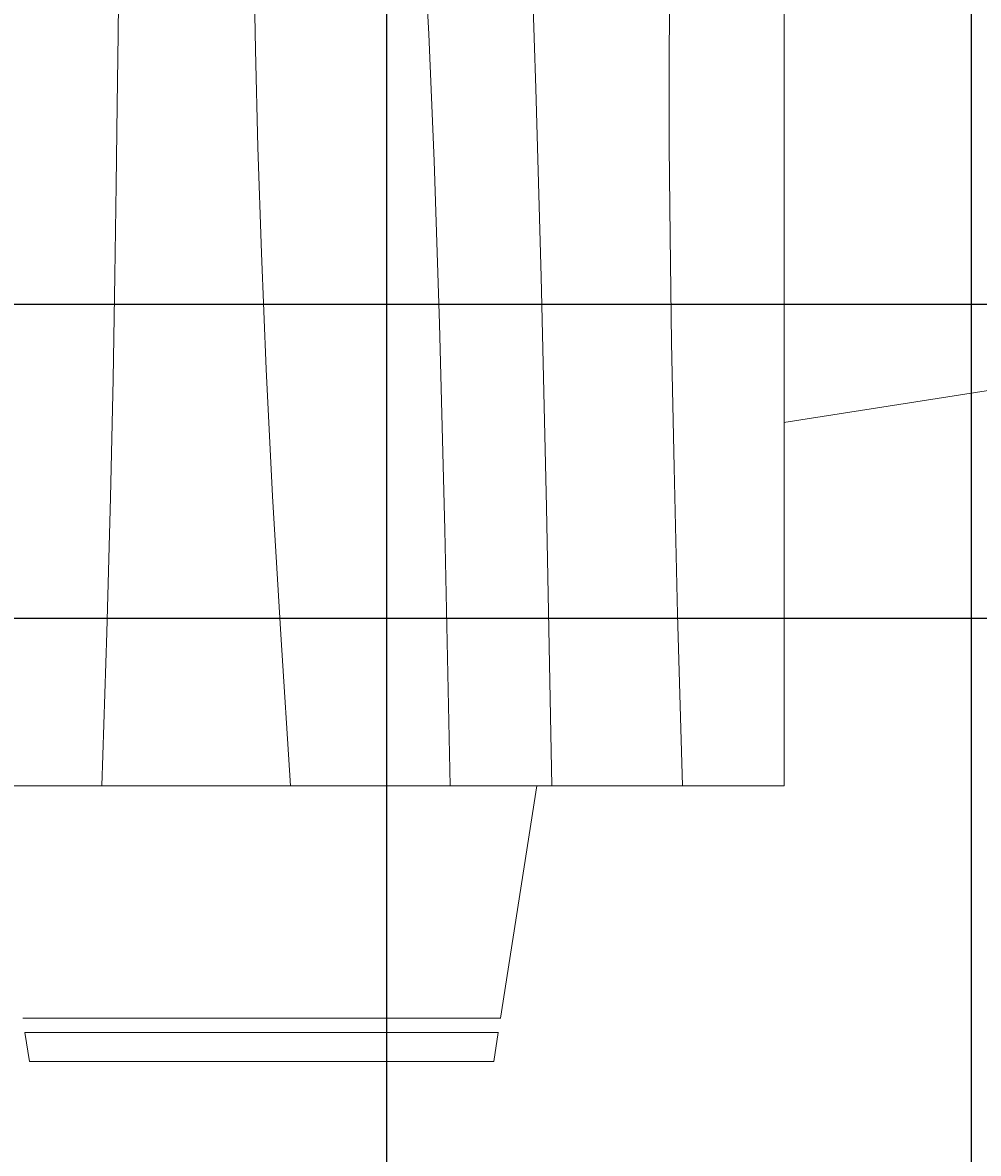
# Model space of a CAD drawing. Units: feet. Extents: x 1654 to 2985, y 1348 to 2230.
# Tile 26 of 53: x 1985 to 2014, y 1785 to 1820. Entities that reach past the tile are written whole.
import ezdxf

# ---------------------------------------------------------------- set-up
doc = ezdxf.new("R2010")
doc.units = ezdxf.units.FT
doc.layers.add('A-ANNO-DIMS', color=2, linetype='Continuous', lineweight=18)
doc.layers.add('A-FURN', color=8, linetype='Continuous', lineweight=13)
doc.styles.get("Standard").update_dxf_attribs({"font": 'arial.ttf'})
doc.dimstyles.get("Standard").update_dxf_attribs({"dimtxt": 0.18, "dimasz": 0.18, "dimexe": 0.18, "dimexo": 0.0625, "dimgap": 0.09, "dimtad": 0, "dimtih": 1, "dimtoh": 1, "dimdec": 4, "dimzin": 0, "dimdsep": 46, "dimtxsty": 'Standard', "dimcen": 0.09, "dimadec": 0, "dimazin": 0, "dimtfac": 1, "dimtdec": 4, "dimtofl": 0, "dimtmove": 0, "dimatfit": 3, "dimfxl": 1, "dimtolj": 1, "dimtzin": 0, "dimarcsym": 0})

# ---------------------------------------------------------------- blocks, each defined once
blk = doc.blocks.new('Dining Set - 36 x 72 in.')
for p, q in [((-36, 18), (-36, -18)), ((-44, 8.23041), (-44, -8.23915)), ((-45.5, 8), (-44.5004, 8.15617)), ((-45.5, 8), (-45.5, -8)), ((-44.5, -8.15843), (-44.5, 8.15338)), ((-44.4997, -8.15631), (-45.5, -8)), ((-35.9976, -9.48476), (-43.9993, -8.2345)), ((-36, -18), (36, -18)), ((-22.2343, -26.0006), (-23.4847, -17.99762))]:
    blk.add_line(p, q)
for points in [[(-36, 5.5), (-30.7157, 5.3348), (-26.069, 5.20963), (-21.9946, 5.11767), (-18.4271, 5.05208), (-15.3009, 5.00602), (-12.5508, 4.97265), (-10.1112, 4.94515), (-7.9167, 4.91666)], [(-36, -1), (-30.7915, -0.6591), (-26.0195, -0.38216), (-21.6519, -0.16284), (-17.6563, 0.00521), (-14.0005, 0.12833), (-10.6523, 0.21289), (-7.5796, 0.26522)], [(-36, -6.5), (-27.1843, -6.31267), (-20.084, -6.1263), (-14.469, -5.9419), (-10.1094, -5.76042), (-6.7752, -5.58285)], [(-36, -10), (-26.4022, -9.81299), (-18.4675, -9.62891), (-11.9839, -9.45069), (-6.7396, -9.28125)], [(-36, -14.5), (-30.0881, -14.33513), (-25.0332, -14.21224), (-20.7312, -14.12647), (-17.0781, -14.07292), (-13.97, -14.04671), (-11.3027, -14.04297), (-8.9724, -14.05681)]]:
    blk.add_lwpolyline(points)
blk = doc.blocks.new('*D91')
at = {"layer": 'A-ANNO-DIMS', "color": 0, "lineweight": -2, "transparency": 16777216}
for p, q in [((1852.155, 1801.468), (2242.272, 1801.468)), ((2242.092, 1801.288), (2242.092, 1776.544)), ((2242.092, 1751.435), (2242.092, 1776.18)), ((1852.155, 1751.255), (2242.272, 1751.255))]:
    blk.add_line(p, q, dxfattribs=at)
at = {"layer": 'A-ANNO-DIMS', "color": 0, "transparency": 16777216}
for points in [[(2242.062, 1801.288), (2242.122, 1801.288), (2242.092, 1801.468)], [(2242.062, 1751.435), (2242.122, 1751.435), (2242.092, 1751.255)]]:
    blk.add_solid(points, dxfattribs=at)
at = {"layer": 'Defpoints', "color": 0, "transparency": 16777216}
for p in [(1852.092, 1801.468), (2242.092, 1801.468), (1852.092, 1751.255)]:
    blk.add_point(p, dxfattribs=at)
at = {"layer": 'A-ANNO-DIMS', "color": 0, "transparency": 16777216, "insert": (2242.092, 1776.362), "char_height": 0.18, "attachment_point": 5}
blk.add_mtext('\\A1;50.21', dxfattribs=at)
blk = doc.blocks.new('*D98')
at = {"layer": 'A-ANNO-DIMS', "color": 0, "lineweight": -2, "transparency": 16777216}
for p, q in [((2061.03, 1811.081), (1811.912, 1811.081)), ((1812.092, 1810.901), (1812.092, 1781.35)), ((1812.092, 1751.435), (1812.092, 1780.986)), ((2061.03, 1751.255), (1811.912, 1751.255))]:
    blk.add_line(p, q, dxfattribs=at)
at = {"layer": 'A-ANNO-DIMS', "color": 0, "transparency": 16777216}
for points in [[(1812.062, 1810.901), (1812.122, 1810.901), (1812.092, 1811.081)], [(1812.062, 1751.435), (1812.122, 1751.435), (1812.092, 1751.255)]]:
    blk.add_solid(points, dxfattribs=at)
at = {"layer": 'Defpoints', "color": 0, "transparency": 16777216}
for p in [(1812.092, 1811.081), (2061.092, 1811.081), (2061.092, 1751.255)]:
    blk.add_point(p, dxfattribs=at)
at = {"layer": 'A-ANNO-DIMS', "color": 0, "transparency": 16777216, "insert": (1812.092, 1781.168), "char_height": 0.18, "attachment_point": 5}
blk.add_mtext('\\A1;59.83', dxfattribs=at)
blk = doc.blocks.new('*D101')
at = {"layer": 'A-ANNO-DIMS', "color": 0, "lineweight": -2, "transparency": 16777216}
for p, q in [((1996.092, 2039.192), (1996.092, 1534.075)), ((2014.016, 2039.192), (2014.016, 1534.075)), ((1996.272, 1534.255), (2004.599, 1534.255)), ((2013.836, 1534.255), (2005.509, 1534.255))]:
    blk.add_line(p, q, dxfattribs=at)
at = {"layer": 'A-ANNO-DIMS', "color": 0, "transparency": 16777216}
for points in [[(1996.272, 1534.285), (1996.272, 1534.225), (1996.092, 1534.255)], [(2013.836, 1534.285), (2013.836, 1534.225), (2014.016, 1534.255)]]:
    blk.add_solid(points, dxfattribs=at)
at = {"layer": 'Defpoints', "color": 0, "transparency": 16777216}
for p in [(1996.092, 2039.255), (2014.016, 2039.255), (2014.016, 1534.255)]:
    blk.add_point(p, dxfattribs=at)
at = {"layer": 'A-ANNO-DIMS', "color": 0, "transparency": 16777216, "insert": (2005.054, 1534.255), "char_height": 0.18, "attachment_point": 5}
blk.add_mtext('\\A1;17.924', dxfattribs=at)

msp = doc.modelspace()

# ---------------------------------------------------------------- block references
at = {"layer": 'A-FURN', "xscale": 0.8893748792417884, "yscale": 0.8893748792417884, "zscale": 0.8893748792417884, "rotation": 90}
msp.add_blockref('Dining Set - 36 x 72 in.', (1992.2681, 1828.3522), dxfattribs=at)

# ---------------------------------------------------------------- dimensions: what is measured, and where the dimension line sits
at = {"layer": 'A-ANNO-DIMS'}
dim = msp.add_linear_dim(base=(2014.016, 1534.2549), p1=(1996.0924, 2039.2549), p2=(2014.016, 2039.2549), dimstyle='Standard', override={"dimdec": 3, "dimlfac": 1, "dimrnd": 0, "dimzin": 0, "dimdsep": 46, "dimlunit": 2}, dxfattribs=at)
dim.commit()
dim.dimension.update_dxf_attribs({"geometry": '*D101', "text_midpoint": (2005.0542, 1534.2549)})
for base, p1, p2, picture, middle in [((1812.0924, 1811.0815), (2061.0924, 1751.2549), (2061.0924, 1811.0815), '*D98', (1812.0924, 1781.1682)), ((2242.0924, 1801.4683), (1852.0924, 1751.2549), (1852.0924, 1801.4683), '*D91', (2242.0924, 1776.3616))]:
    dim = msp.add_linear_dim(base=base, p1=p1, p2=p2, angle=90, dimstyle='Standard', override={"dimdec": 2, "dimlfac": 1, "dimrnd": 0, "dimzin": 0, "dimdsep": 46, "dimlunit": 2}, dxfattribs=at)
    dim.commit()
    dim.dimension.update_dxf_attribs({"geometry": picture, "text_midpoint": middle})

doc.saveas('drawing.dxf')
